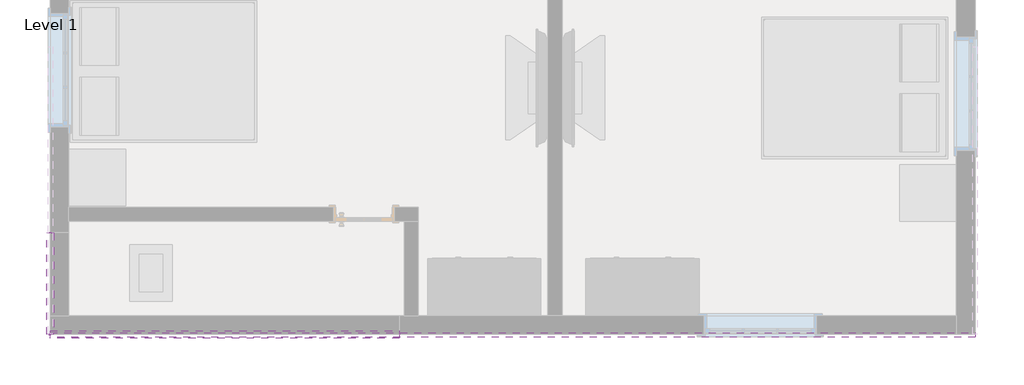
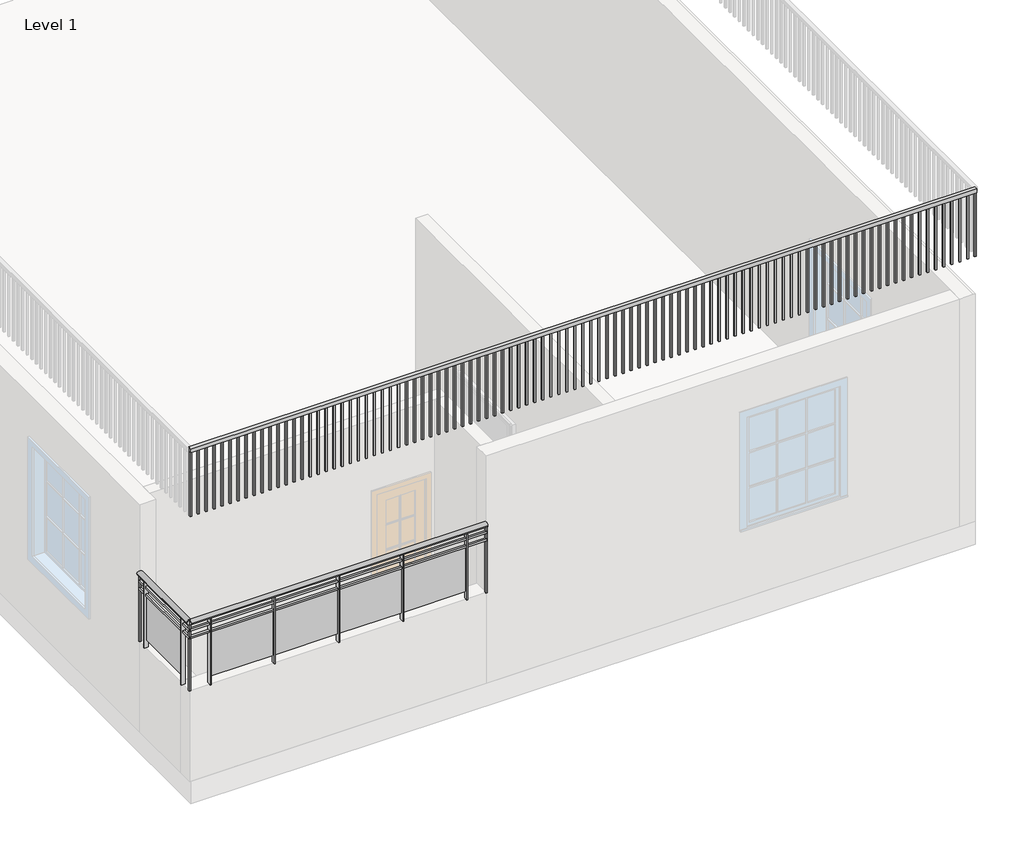
# One storey, part 2 of 7: 3 railings.
"""IFC4 building model written with IfcOpenShell, lengths in millimetres."""

from ifc_helpers import new_model, si_unit, point, frame, origin, place, context, project, spatial, polyline, ellipse_curve, trimmed, outline, extrude, element, save
from ifc_brep_helpers import plane_surface, extruded_surface, advanced_brep

model = new_model("IFC4")

# Units and contexts
model_context = context("Model", 3, world=origin())
ifc_project = project(units=[si_unit("LENGTHUNIT", "METRE", prefix="MILLI")], contexts=[model_context])

# Site, building, storey
site = spatial("IfcSite", under=ifc_project)
building = spatial("IfcBuilding", under=site)
storey = spatial("IfcBuildingStorey", under=building, Name="Level 1", Elevation=0.0)

# Railings
placement = place(None, origin())
element("IfcRailing", 1, ObjectType="Glass Panel - Bottom Fill", at=placement, inside=storey, context=model_context, shape_type="SolidModel", body=[
    advanced_brep(
    [(-8442.18475, -376.3160527, 2133.6), (-8518.38475, -376.3160527, 2133.6), (-8442.18475, -1468.5160527, 2133.6), (-8518.38475, -1468.5160527, 2133.6)],
    [
        (0, 1, ellipse_curve(frame((-8480.28475, -376.3160527, 2133.6), z_axis=(0.0, 1.0, 0.0), x_axis=(-1.0, 0.0, 0.0)), 38.1, 28.575)),
        (1, 0, ellipse_curve(frame((-8480.28475, -376.3160527, 2133.6), z_axis=(0.0, 1.0, 0.0), x_axis=(-1.0, 0.0, 0.0)), 38.1, 28.575)),
        (2, 3, ellipse_curve(frame((-8480.28475, -1468.5160527, 2133.6), z_axis=(0.0, -1.0, 0.0), x_axis=(-1.0, 0.0, 0.0)), 38.1, 28.575)),
        (3, 2, ellipse_curve(frame((-8480.28475, -1468.5160527, 2133.6), z_axis=(0.0, -1.0, 0.0), x_axis=(-1.0, 0.0, 0.0)), 38.1, 28.575)),
        (0, 2),
        (3, 1),
    ],
    [
        plane_surface(frame((-8480.28475, -376.3160527, 2133.6), z_axis=(0.0, 1.0, 0.0), x_axis=(0.0, 0.0, -1.0))),
        plane_surface(frame((-8480.28475, -1468.5160527, 2133.6), z_axis=(0.0, -1.0, 0.0), x_axis=(0.0, 0.0, -1.0))),
        extruded_surface(trimmed(ellipse_curve(frame((-8480.28475, -1468.5160527, 2133.6), z_axis=(0.0, 1.0, 0.0), x_axis=(-1.0, 0.0, 0.0)), 38.1, 28.575), [point((-8442.18475, -1468.5160527, 2133.6))], [point((-8518.38475, -1468.5160527, 2133.6))], True, "CARTESIAN"), (0.0, 1092.2, 0.0), 1092.2),
        extruded_surface(trimmed(ellipse_curve(frame((-8480.28475, -1468.5160527, 2133.6), z_axis=(0.0, 1.0, 0.0), x_axis=(-1.0, 0.0, 0.0)), 38.1, 28.575), [point((-8518.38475, -1468.5160527, 2133.6))], [point((-8442.18475, -1468.5160527, 2133.6))], True, "CARTESIAN"), (0.0, 1092.2, 0.0), 1092.2),
    ],
    [
        (0, [[1, 2]]),
        (1, [[3, 4]]),
        (2, [[-1, 5, -4, 6]]),
        (3, [[-2, -6, -3, -5]]),
    ],
),
    extrude(outline(polyline([(-8492.98475, -376.3160527), (-8467.58475, -376.3160527), (-8467.58475, -1468.5160527), (-8492.98475, -1468.5160527), (-8492.98475, -376.3160527)])), frame((0.0, 0.0, 2019.3), z_axis=(0.0, 0.0, 1.0), x_axis=(1.0, 0.0, 0.0)), (0.0, 0.0, 1.0), 25.4),
    extrude(outline(polyline([(-8492.98475, -376.3160527), (-8467.58475, -376.3160527), (-8467.58475, -1468.5160527), (-8492.98475, -1468.5160527), (-8492.98475, -376.3160527)])), frame((0.0, 0.0, 1917.7), z_axis=(0.0, 0.0, 1.0), x_axis=(1.0, 0.0, 0.0)), (0.0, 0.0, 1.0), 25.4),
    extrude(outline(polyline([(-8505.68475, -1322.4660527), (-8454.88475, -1322.4660527), (-8454.88475, -1335.1660527), (-8505.68475, -1335.1660527), (-8505.68475, -1322.4660527)])), frame((0.0, 0.0, 1219.2), z_axis=(0.0, 0.0, 1.0), x_axis=(1.0, 0.0, 0.0)), (0.0, 0.0, 1.0), 885.6788223),
    extrude(outline(polyline([(-8473.749593, -516.0160527), (-8473.749593, -1328.8160527), (-8480.099593, -1328.8160527), (-8480.099593, -516.0160527), (-8473.749593, -516.0160527)])), frame((0.0, 0.0, 1320.8), z_axis=(0.0, 0.0, 1.0), x_axis=(1.0, 0.0, 0.0)), (0.0, 0.0, 1.0), 596.9),
    extrude(outline(polyline([(-8505.68475, -509.6660527), (-8454.88475, -509.6660527), (-8454.88475, -522.3660527), (-8505.68475, -522.3660527), (-8505.68475, -509.6660527)])), frame((0.0, 0.0, 1219.2), z_axis=(0.0, 0.0, 1.0), x_axis=(1.0, 0.0, 0.0)), (0.0, 0.0, 1.0), 885.6788223),
    extrude(outline(polyline([(-8489.80975, -1455.8160527), (-8470.75975, -1455.8160527), (-8470.75975, -1474.8660527), (-8489.80975, -1474.8660527), (-8489.80975, -1455.8160527)])), frame((0.0, 0.0, 1219.2), z_axis=(0.0, 0.0, 1.0), x_axis=(1.0, 0.0, 0.0)), (0.0, 0.0, 1.0), 885.6788223),
    extrude(outline(polyline([(-8489.80975, -369.9660527), (-8470.75975, -369.9660527), (-8470.75975, -389.0160527), (-8489.80975, -389.0160527), (-8489.80975, -369.9660527)])), frame((0.0, 0.0, 1219.2), z_axis=(0.0, 0.0, 1.0), x_axis=(1.0, 0.0, 0.0)), (0.0, 0.0, 1.0), 885.6788223),
])
element("IfcRailing", 2, ObjectType="Glass Panel - Bottom Fill", at=placement, inside=storey, context=model_context, shape_type="SolidModel", body=[
    advanced_brep(
    [(-8480.28475, -1430.4160527, 2133.6), (-8480.28475, -1506.6160527, 2133.6), (-4721.08475, -1430.4160527, 2133.6), (-4721.08475, -1506.6160527, 2133.6)],
    [
        (0, 1, ellipse_curve(frame((-8480.28475, -1468.5160527, 2133.6), z_axis=(-1.0, 0.0, 0.0), x_axis=(0.0, -1.0, 0.0)), 38.1, 28.575)),
        (1, 0, ellipse_curve(frame((-8480.28475, -1468.5160527, 2133.6), z_axis=(-1.0, 0.0, 0.0), x_axis=(0.0, -1.0, 0.0)), 38.1, 28.575)),
        (2, 3, ellipse_curve(frame((-4721.08475, -1468.5160527, 2133.6), z_axis=(1.0, 0.0, 0.0), x_axis=(0.0, -1.0, 0.0)), 38.1, 28.575)),
        (3, 2, ellipse_curve(frame((-4721.08475, -1468.5160527, 2133.6), z_axis=(1.0, 0.0, 0.0), x_axis=(0.0, -1.0, 0.0)), 38.1, 28.575)),
        (0, 2),
        (3, 1),
    ],
    [
        plane_surface(frame((-8480.28475, -1468.5160527, 2133.6), z_axis=(-1.0, 0.0, 0.0), x_axis=(0.0, 1.0, 0.0))),
        plane_surface(frame((-4721.08475, -1468.5160527, 2133.6), z_axis=(1.0, 0.0, 0.0), x_axis=(0.0, 1.0, 0.0))),
        extruded_surface(trimmed(ellipse_curve(frame((-4721.08475, -1468.5160527, 2133.6), z_axis=(-1.0, 0.0, 0.0), x_axis=(0.0, -1.0, 0.0)), 38.1, 28.575), [point((-4721.08475, -1430.4160527, 2133.6))], [point((-4721.08475, -1506.6160527, 2133.6))], True, "CARTESIAN"), (-3759.2000000000007, 0.0, 0.0), 3759.2000000000007),
        extruded_surface(trimmed(ellipse_curve(frame((-4721.08475, -1468.5160527, 2133.6), z_axis=(-1.0, 0.0, 0.0), x_axis=(0.0, -1.0, 0.0)), 38.1, 28.575), [point((-4721.08475, -1506.6160527, 2133.6))], [point((-4721.08475, -1430.4160527, 2133.6))], True, "CARTESIAN"), (-3759.2000000000007, 0.0, 0.0), 3759.2000000000007),
    ],
    [
        (0, [[1, 2]]),
        (1, [[3, 4]]),
        (2, [[-1, 5, -4, 6]]),
        (3, [[-2, -6, -3, -5]]),
    ],
),
    extrude(outline(polyline([(-8480.28475, -1481.2160527), (-8480.28475, -1455.8160527), (-4721.08475, -1455.8160527), (-4721.08475, -1481.2160527), (-8480.28475, -1481.2160527)])), frame((0.0, 0.0, 2019.3), z_axis=(0.0, 0.0, 1.0), x_axis=(1.0, 0.0, 0.0)), (0.0, 0.0, 1.0), 25.4),
    extrude(outline(polyline([(-8480.28475, -1481.2160527), (-8480.28475, -1455.8160527), (-4721.08475, -1455.8160527), (-4721.08475, -1481.2160527), (-8480.28475, -1481.2160527)])), frame((0.0, 0.0, 1917.7), z_axis=(0.0, 0.0, 1.0), x_axis=(1.0, 0.0, 0.0)), (0.0, 0.0, 1.0), 25.4),
    extrude(outline(polyline([(-4981.43475, -1493.9160527), (-4981.43475, -1443.1160527), (-4968.73475, -1443.1160527), (-4968.73475, -1493.9160527), (-4981.43475, -1493.9160527)])), frame((0.0, 0.0, 1219.2), z_axis=(0.0, 0.0, 1.0), x_axis=(1.0, 0.0, 0.0)), (0.0, 0.0, 1.0), 885.6788223),
    extrude(outline(polyline([(-5787.88475, -1461.9808957), (-4975.08475, -1461.9808957), (-4975.08475, -1468.3308957), (-5787.88475, -1468.3308957), (-5787.88475, -1461.9808957)])), frame((0.0, 0.0, 1320.8), z_axis=(0.0, 0.0, 1.0), x_axis=(1.0, 0.0, 0.0)), (0.0, 0.0, 1.0), 596.9),
    extrude(outline(polyline([(-5794.23475, -1493.9160527), (-5794.23475, -1443.1160527), (-5781.53475, -1443.1160527), (-5781.53475, -1493.9160527), (-5794.23475, -1493.9160527)])), frame((0.0, 0.0, 1219.2), z_axis=(0.0, 0.0, 1.0), x_axis=(1.0, 0.0, 0.0)), (0.0, 0.0, 1.0), 885.6788223),
    extrude(outline(polyline([(-6600.68475, -1461.9808957), (-5787.88475, -1461.9808957), (-5787.88475, -1468.3308957), (-6600.68475, -1468.3308957), (-6600.68475, -1461.9808957)])), frame((0.0, 0.0, 1320.8), z_axis=(0.0, 0.0, 1.0), x_axis=(1.0, 0.0, 0.0)), (0.0, 0.0, 1.0), 596.9),
    extrude(outline(polyline([(-6607.03475, -1493.9160527), (-6607.03475, -1443.1160527), (-6594.33475, -1443.1160527), (-6594.33475, -1493.9160527), (-6607.03475, -1493.9160527)])), frame((0.0, 0.0, 1219.2), z_axis=(0.0, 0.0, 1.0), x_axis=(1.0, 0.0, 0.0)), (0.0, 0.0, 1.0), 885.6788223),
    extrude(outline(polyline([(-7413.48475, -1461.9808957), (-6600.68475, -1461.9808957), (-6600.68475, -1468.3308957), (-7413.48475, -1468.3308957), (-7413.48475, -1461.9808957)])), frame((0.0, 0.0, 1320.8), z_axis=(0.0, 0.0, 1.0), x_axis=(1.0, 0.0, 0.0)), (0.0, 0.0, 1.0), 596.9),
    extrude(outline(polyline([(-7419.83475, -1493.9160527), (-7419.83475, -1443.1160527), (-7407.13475, -1443.1160527), (-7407.13475, -1493.9160527), (-7419.83475, -1493.9160527)])), frame((0.0, 0.0, 1219.2), z_axis=(0.0, 0.0, 1.0), x_axis=(1.0, 0.0, 0.0)), (0.0, 0.0, 1.0), 885.6788223),
    extrude(outline(polyline([(-8226.28475, -1461.9808957), (-7413.48475, -1461.9808957), (-7413.48475, -1468.3308957), (-8226.28475, -1468.3308957), (-8226.28475, -1461.9808957)])), frame((0.0, 0.0, 1320.8), z_axis=(0.0, 0.0, 1.0), x_axis=(1.0, 0.0, 0.0)), (0.0, 0.0, 1.0), 596.9),
    extrude(outline(polyline([(-8232.63475, -1493.9160527), (-8232.63475, -1443.1160527), (-8219.93475, -1443.1160527), (-8219.93475, -1493.9160527), (-8232.63475, -1493.9160527)])), frame((0.0, 0.0, 1219.2), z_axis=(0.0, 0.0, 1.0), x_axis=(1.0, 0.0, 0.0)), (0.0, 0.0, 1.0), 885.6788223),
    extrude(outline(polyline([(-4733.78475, -1478.0410527), (-4733.78475, -1458.9910527), (-4714.73475, -1458.9910527), (-4714.73475, -1478.0410527), (-4733.78475, -1478.0410527)])), frame((0.0, 0.0, 1219.2), z_axis=(0.0, 0.0, 1.0), x_axis=(1.0, 0.0, 0.0)), (0.0, 0.0, 1.0), 885.6788223),
    extrude(outline(polyline([(-8486.63475, -1478.0410527), (-8486.63475, -1458.9910527), (-8467.58475, -1458.9910527), (-8467.58475, -1478.0410527), (-8486.63475, -1478.0410527)])), frame((0.0, 0.0, 1219.2), z_axis=(0.0, 0.0, 1.0), x_axis=(1.0, 0.0, 0.0)), (0.0, 0.0, 1.0), 885.6788223),
])
element("IfcRailing", 3, ObjectType="Handrail - Rectangular", at=placement, inside=storey, context=model_context, shape_type="SweptSolid", body=[
    extrude(outline(polyline([(-8480.28475, -1500.2660527), (-8480.28475, -1449.4660527), (1476.51525, -1449.4660527), (1476.51525, -1500.2660527), (-8480.28475, -1500.2660527)])), frame((0.0, 0.0, 4419.6), z_axis=(0.0, 0.0, 1.0), x_axis=(1.0, 0.0, 0.0)), (0.0, 0.0, 1.0), 50.8),
    extrude(outline(polyline([(1365.39025, -1484.3910527), (1365.39025, -1465.3410527), (1384.44025, -1465.3410527), (1384.44025, -1484.3910527), (1365.39025, -1484.3910527)])), frame((0.0, 0.0, 3556.0), z_axis=(0.0, 0.0, 1.0), x_axis=(1.0, 0.0, 0.0)), (0.0, 0.0, 1.0), 863.6),
    extrude(outline(polyline([(1263.79025, -1484.3910527), (1263.79025, -1465.3410527), (1282.84025, -1465.3410527), (1282.84025, -1484.3910527), (1263.79025, -1484.3910527)])), frame((0.0, 0.0, 3556.0), z_axis=(0.0, 0.0, 1.0), x_axis=(1.0, 0.0, 0.0)), (0.0, 0.0, 1.0), 863.6),
    extrude(outline(polyline([(1162.19025, -1484.3910527), (1162.19025, -1465.3410527), (1181.24025, -1465.3410527), (1181.24025, -1484.3910527), (1162.19025, -1484.3910527)])), frame((0.0, 0.0, 3556.0), z_axis=(0.0, 0.0, 1.0), x_axis=(1.0, 0.0, 0.0)), (0.0, 0.0, 1.0), 863.6),
    extrude(outline(polyline([(1060.59025, -1484.3910527), (1060.59025, -1465.3410527), (1079.64025, -1465.3410527), (1079.64025, -1484.3910527), (1060.59025, -1484.3910527)])), frame((0.0, 0.0, 3556.0), z_axis=(0.0, 0.0, 1.0), x_axis=(1.0, 0.0, 0.0)), (0.0, 0.0, 1.0), 863.6),
    extrude(outline(polyline([(958.99025, -1484.3910527), (958.99025, -1465.3410527), (978.04025, -1465.3410527), (978.04025, -1484.3910527), (958.99025, -1484.3910527)])), frame((0.0, 0.0, 3556.0), z_axis=(0.0, 0.0, 1.0), x_axis=(1.0, 0.0, 0.0)), (0.0, 0.0, 1.0), 863.6),
    extrude(outline(polyline([(857.39025, -1484.3910527), (857.39025, -1465.3410527), (876.44025, -1465.3410527), (876.44025, -1484.3910527), (857.39025, -1484.3910527)])), frame((0.0, 0.0, 3556.0), z_axis=(0.0, 0.0, 1.0), x_axis=(1.0, 0.0, 0.0)), (0.0, 0.0, 1.0), 863.6),
    extrude(outline(polyline([(755.79025, -1484.3910527), (755.79025, -1465.3410527), (774.84025, -1465.3410527), (774.84025, -1484.3910527), (755.79025, -1484.3910527)])), frame((0.0, 0.0, 3556.0), z_axis=(0.0, 0.0, 1.0), x_axis=(1.0, 0.0, 0.0)), (0.0, 0.0, 1.0), 863.6),
    extrude(outline(polyline([(654.19025, -1484.3910527), (654.19025, -1465.3410527), (673.24025, -1465.3410527), (673.24025, -1484.3910527), (654.19025, -1484.3910527)])), frame((0.0, 0.0, 3556.0), z_axis=(0.0, 0.0, 1.0), x_axis=(1.0, 0.0, 0.0)), (0.0, 0.0, 1.0), 863.6),
    extrude(outline(polyline([(552.59025, -1484.3910527), (552.59025, -1465.3410527), (571.64025, -1465.3410527), (571.64025, -1484.3910527), (552.59025, -1484.3910527)])), frame((0.0, 0.0, 3556.0), z_axis=(0.0, 0.0, 1.0), x_axis=(1.0, 0.0, 0.0)), (0.0, 0.0, 1.0), 863.6),
    extrude(outline(polyline([(450.99025, -1484.3910527), (450.99025, -1465.3410527), (470.04025, -1465.3410527), (470.04025, -1484.3910527), (450.99025, -1484.3910527)])), frame((0.0, 0.0, 3556.0), z_axis=(0.0, 0.0, 1.0), x_axis=(1.0, 0.0, 0.0)), (0.0, 0.0, 1.0), 863.6),
    extrude(outline(polyline([(349.39025, -1484.3910527), (349.39025, -1465.3410527), (368.44025, -1465.3410527), (368.44025, -1484.3910527), (349.39025, -1484.3910527)])), frame((0.0, 0.0, 3556.0), z_axis=(0.0, 0.0, 1.0), x_axis=(1.0, 0.0, 0.0)), (0.0, 0.0, 1.0), 863.6),
    extrude(outline(polyline([(247.79025, -1484.3910527), (247.79025, -1465.3410527), (266.84025, -1465.3410527), (266.84025, -1484.3910527), (247.79025, -1484.3910527)])), frame((0.0, 0.0, 3556.0), z_axis=(0.0, 0.0, 1.0), x_axis=(1.0, 0.0, 0.0)), (0.0, 0.0, 1.0), 863.6),
    extrude(outline(polyline([(146.19025, -1484.3910527), (146.19025, -1465.3410527), (165.24025, -1465.3410527), (165.24025, -1484.3910527), (146.19025, -1484.3910527)])), frame((0.0, 0.0, 3556.0), z_axis=(0.0, 0.0, 1.0), x_axis=(1.0, 0.0, 0.0)), (0.0, 0.0, 1.0), 863.6),
    extrude(outline(polyline([(44.59025, -1484.3910527), (44.59025, -1465.3410527), (63.64025, -1465.3410527), (63.64025, -1484.3910527), (44.59025, -1484.3910527)])), frame((0.0, 0.0, 3556.0), z_axis=(0.0, 0.0, 1.0), x_axis=(1.0, 0.0, 0.0)), (0.0, 0.0, 1.0), 863.6),
    extrude(outline(polyline([(-57.00975, -1484.3910527), (-57.00975, -1465.3410527), (-37.95975, -1465.3410527), (-37.95975, -1484.3910527), (-57.00975, -1484.3910527)])), frame((0.0, 0.0, 3556.0), z_axis=(0.0, 0.0, 1.0), x_axis=(1.0, 0.0, 0.0)), (0.0, 0.0, 1.0), 863.6),
    extrude(outline(polyline([(-158.60975, -1484.3910527), (-158.60975, -1465.3410527), (-139.55975, -1465.3410527), (-139.55975, -1484.3910527), (-158.60975, -1484.3910527)])), frame((0.0, 0.0, 3556.0), z_axis=(0.0, 0.0, 1.0), x_axis=(1.0, 0.0, 0.0)), (0.0, 0.0, 1.0), 863.6),
    extrude(outline(polyline([(-260.20975, -1484.3910527), (-260.20975, -1465.3410527), (-241.15975, -1465.3410527), (-241.15975, -1484.3910527), (-260.20975, -1484.3910527)])), frame((0.0, 0.0, 3556.0), z_axis=(0.0, 0.0, 1.0), x_axis=(1.0, 0.0, 0.0)), (0.0, 0.0, 1.0), 863.6),
    extrude(outline(polyline([(-361.80975, -1484.3910527), (-361.80975, -1465.3410527), (-342.75975, -1465.3410527), (-342.75975, -1484.3910527), (-361.80975, -1484.3910527)])), frame((0.0, 0.0, 3556.0), z_axis=(0.0, 0.0, 1.0), x_axis=(1.0, 0.0, 0.0)), (0.0, 0.0, 1.0), 863.6),
    extrude(outline(polyline([(-463.40975, -1484.3910527), (-463.40975, -1465.3410527), (-444.35975, -1465.3410527), (-444.35975, -1484.3910527), (-463.40975, -1484.3910527)])), frame((0.0, 0.0, 3556.0), z_axis=(0.0, 0.0, 1.0), x_axis=(1.0, 0.0, 0.0)), (0.0, 0.0, 1.0), 863.6),
    extrude(outline(polyline([(-565.00975, -1484.3910527), (-565.00975, -1465.3410527), (-545.95975, -1465.3410527), (-545.95975, -1484.3910527), (-565.00975, -1484.3910527)])), frame((0.0, 0.0, 3556.0), z_axis=(0.0, 0.0, 1.0), x_axis=(1.0, 0.0, 0.0)), (0.0, 0.0, 1.0), 863.6),
    extrude(outline(polyline([(-666.60975, -1484.3910527), (-666.60975, -1465.3410527), (-647.55975, -1465.3410527), (-647.55975, -1484.3910527), (-666.60975, -1484.3910527)])), frame((0.0, 0.0, 3556.0), z_axis=(0.0, 0.0, 1.0), x_axis=(1.0, 0.0, 0.0)), (0.0, 0.0, 1.0), 863.6),
    extrude(outline(polyline([(-768.20975, -1484.3910527), (-768.20975, -1465.3410527), (-749.15975, -1465.3410527), (-749.15975, -1484.3910527), (-768.20975, -1484.3910527)])), frame((0.0, 0.0, 3556.0), z_axis=(0.0, 0.0, 1.0), x_axis=(1.0, 0.0, 0.0)), (0.0, 0.0, 1.0), 863.6),
    extrude(outline(polyline([(-869.80975, -1484.3910527), (-869.80975, -1465.3410527), (-850.75975, -1465.3410527), (-850.75975, -1484.3910527), (-869.80975, -1484.3910527)])), frame((0.0, 0.0, 3556.0), z_axis=(0.0, 0.0, 1.0), x_axis=(1.0, 0.0, 0.0)), (0.0, 0.0, 1.0), 863.6),
    extrude(outline(polyline([(-971.40975, -1484.3910527), (-971.40975, -1465.3410527), (-952.35975, -1465.3410527), (-952.35975, -1484.3910527), (-971.40975, -1484.3910527)])), frame((0.0, 0.0, 3556.0), z_axis=(0.0, 0.0, 1.0), x_axis=(1.0, 0.0, 0.0)), (0.0, 0.0, 1.0), 863.6),
    extrude(outline(polyline([(-1073.00975, -1484.3910527), (-1073.00975, -1465.3410527), (-1053.95975, -1465.3410527), (-1053.95975, -1484.3910527), (-1073.00975, -1484.3910527)])), frame((0.0, 0.0, 3556.0), z_axis=(0.0, 0.0, 1.0), x_axis=(1.0, 0.0, 0.0)), (0.0, 0.0, 1.0), 863.6),
    extrude(outline(polyline([(-1174.60975, -1484.3910527), (-1174.60975, -1465.3410527), (-1155.55975, -1465.3410527), (-1155.55975, -1484.3910527), (-1174.60975, -1484.3910527)])), frame((0.0, 0.0, 3556.0), z_axis=(0.0, 0.0, 1.0), x_axis=(1.0, 0.0, 0.0)), (0.0, 0.0, 1.0), 863.6),
    extrude(outline(polyline([(-1276.20975, -1484.3910527), (-1276.20975, -1465.3410527), (-1257.15975, -1465.3410527), (-1257.15975, -1484.3910527), (-1276.20975, -1484.3910527)])), frame((0.0, 0.0, 3556.0), z_axis=(0.0, 0.0, 1.0), x_axis=(1.0, 0.0, 0.0)), (0.0, 0.0, 1.0), 863.6),
    extrude(outline(polyline([(-1377.80975, -1484.3910527), (-1377.80975, -1465.3410527), (-1358.75975, -1465.3410527), (-1358.75975, -1484.3910527), (-1377.80975, -1484.3910527)])), frame((0.0, 0.0, 3556.0), z_axis=(0.0, 0.0, 1.0), x_axis=(1.0, 0.0, 0.0)), (0.0, 0.0, 1.0), 863.6),
    extrude(outline(polyline([(-1479.40975, -1484.3910527), (-1479.40975, -1465.3410527), (-1460.35975, -1465.3410527), (-1460.35975, -1484.3910527), (-1479.40975, -1484.3910527)])), frame((0.0, 0.0, 3556.0), z_axis=(0.0, 0.0, 1.0), x_axis=(1.0, 0.0, 0.0)), (0.0, 0.0, 1.0), 863.6),
    extrude(outline(polyline([(-1581.00975, -1484.3910527), (-1581.00975, -1465.3410527), (-1561.95975, -1465.3410527), (-1561.95975, -1484.3910527), (-1581.00975, -1484.3910527)])), frame((0.0, 0.0, 3556.0), z_axis=(0.0, 0.0, 1.0), x_axis=(1.0, 0.0, 0.0)), (0.0, 0.0, 1.0), 863.6),
    extrude(outline(polyline([(-1682.60975, -1484.3910527), (-1682.60975, -1465.3410527), (-1663.55975, -1465.3410527), (-1663.55975, -1484.3910527), (-1682.60975, -1484.3910527)])), frame((0.0, 0.0, 3556.0), z_axis=(0.0, 0.0, 1.0), x_axis=(1.0, 0.0, 0.0)), (0.0, 0.0, 1.0), 863.6),
    extrude(outline(polyline([(-1784.20975, -1484.3910527), (-1784.20975, -1465.3410527), (-1765.15975, -1465.3410527), (-1765.15975, -1484.3910527), (-1784.20975, -1484.3910527)])), frame((0.0, 0.0, 3556.0), z_axis=(0.0, 0.0, 1.0), x_axis=(1.0, 0.0, 0.0)), (0.0, 0.0, 1.0), 863.6),
    extrude(outline(polyline([(-1885.80975, -1484.3910527), (-1885.80975, -1465.3410527), (-1866.75975, -1465.3410527), (-1866.75975, -1484.3910527), (-1885.80975, -1484.3910527)])), frame((0.0, 0.0, 3556.0), z_axis=(0.0, 0.0, 1.0), x_axis=(1.0, 0.0, 0.0)), (0.0, 0.0, 1.0), 863.6),
    extrude(outline(polyline([(-1987.40975, -1484.3910527), (-1987.40975, -1465.3410527), (-1968.35975, -1465.3410527), (-1968.35975, -1484.3910527), (-1987.40975, -1484.3910527)])), frame((0.0, 0.0, 3556.0), z_axis=(0.0, 0.0, 1.0), x_axis=(1.0, 0.0, 0.0)), (0.0, 0.0, 1.0), 863.6),
    extrude(outline(polyline([(-2089.00975, -1484.3910527), (-2089.00975, -1465.3410527), (-2069.95975, -1465.3410527), (-2069.95975, -1484.3910527), (-2089.00975, -1484.3910527)])), frame((0.0, 0.0, 3556.0), z_axis=(0.0, 0.0, 1.0), x_axis=(1.0, 0.0, 0.0)), (0.0, 0.0, 1.0), 863.6),
    extrude(outline(polyline([(-2190.60975, -1484.3910527), (-2190.60975, -1465.3410527), (-2171.55975, -1465.3410527), (-2171.55975, -1484.3910527), (-2190.60975, -1484.3910527)])), frame((0.0, 0.0, 3556.0), z_axis=(0.0, 0.0, 1.0), x_axis=(1.0, 0.0, 0.0)), (0.0, 0.0, 1.0), 863.6),
    extrude(outline(polyline([(-2292.20975, -1484.3910527), (-2292.20975, -1465.3410527), (-2273.15975, -1465.3410527), (-2273.15975, -1484.3910527), (-2292.20975, -1484.3910527)])), frame((0.0, 0.0, 3556.0), z_axis=(0.0, 0.0, 1.0), x_axis=(1.0, 0.0, 0.0)), (0.0, 0.0, 1.0), 863.6),
    extrude(outline(polyline([(-2393.80975, -1484.3910527), (-2393.80975, -1465.3410527), (-2374.75975, -1465.3410527), (-2374.75975, -1484.3910527), (-2393.80975, -1484.3910527)])), frame((0.0, 0.0, 3556.0), z_axis=(0.0, 0.0, 1.0), x_axis=(1.0, 0.0, 0.0)), (0.0, 0.0, 1.0), 863.6),
    extrude(outline(polyline([(-2495.40975, -1484.3910527), (-2495.40975, -1465.3410527), (-2476.35975, -1465.3410527), (-2476.35975, -1484.3910527), (-2495.40975, -1484.3910527)])), frame((0.0, 0.0, 3556.0), z_axis=(0.0, 0.0, 1.0), x_axis=(1.0, 0.0, 0.0)), (0.0, 0.0, 1.0), 863.6),
    extrude(outline(polyline([(-2597.00975, -1484.3910527), (-2597.00975, -1465.3410527), (-2577.95975, -1465.3410527), (-2577.95975, -1484.3910527), (-2597.00975, -1484.3910527)])), frame((0.0, 0.0, 3556.0), z_axis=(0.0, 0.0, 1.0), x_axis=(1.0, 0.0, 0.0)), (0.0, 0.0, 1.0), 863.6),
    extrude(outline(polyline([(-2698.60975, -1484.3910527), (-2698.60975, -1465.3410527), (-2679.55975, -1465.3410527), (-2679.55975, -1484.3910527), (-2698.60975, -1484.3910527)])), frame((0.0, 0.0, 3556.0), z_axis=(0.0, 0.0, 1.0), x_axis=(1.0, 0.0, 0.0)), (0.0, 0.0, 1.0), 863.6),
    extrude(outline(polyline([(-2800.20975, -1484.3910527), (-2800.20975, -1465.3410527), (-2781.15975, -1465.3410527), (-2781.15975, -1484.3910527), (-2800.20975, -1484.3910527)])), frame((0.0, 0.0, 3556.0), z_axis=(0.0, 0.0, 1.0), x_axis=(1.0, 0.0, 0.0)), (0.0, 0.0, 1.0), 863.6),
    extrude(outline(polyline([(-2901.80975, -1484.3910527), (-2901.80975, -1465.3410527), (-2882.75975, -1465.3410527), (-2882.75975, -1484.3910527), (-2901.80975, -1484.3910527)])), frame((0.0, 0.0, 3556.0), z_axis=(0.0, 0.0, 1.0), x_axis=(1.0, 0.0, 0.0)), (0.0, 0.0, 1.0), 863.6),
    extrude(outline(polyline([(-3003.40975, -1484.3910527), (-3003.40975, -1465.3410527), (-2984.35975, -1465.3410527), (-2984.35975, -1484.3910527), (-3003.40975, -1484.3910527)])), frame((0.0, 0.0, 3556.0), z_axis=(0.0, 0.0, 1.0), x_axis=(1.0, 0.0, 0.0)), (0.0, 0.0, 1.0), 863.6),
    extrude(outline(polyline([(-3105.00975, -1484.3910527), (-3105.00975, -1465.3410527), (-3085.95975, -1465.3410527), (-3085.95975, -1484.3910527), (-3105.00975, -1484.3910527)])), frame((0.0, 0.0, 3556.0), z_axis=(0.0, 0.0, 1.0), x_axis=(1.0, 0.0, 0.0)), (0.0, 0.0, 1.0), 863.6),
    extrude(outline(polyline([(-3206.60975, -1484.3910527), (-3206.60975, -1465.3410527), (-3187.55975, -1465.3410527), (-3187.55975, -1484.3910527), (-3206.60975, -1484.3910527)])), frame((0.0, 0.0, 3556.0), z_axis=(0.0, 0.0, 1.0), x_axis=(1.0, 0.0, 0.0)), (0.0, 0.0, 1.0), 863.6),
    extrude(outline(polyline([(-3308.20975, -1484.3910527), (-3308.20975, -1465.3410527), (-3289.15975, -1465.3410527), (-3289.15975, -1484.3910527), (-3308.20975, -1484.3910527)])), frame((0.0, 0.0, 3556.0), z_axis=(0.0, 0.0, 1.0), x_axis=(1.0, 0.0, 0.0)), (0.0, 0.0, 1.0), 863.6),
    extrude(outline(polyline([(-3409.80975, -1484.3910527), (-3409.80975, -1465.3410527), (-3390.75975, -1465.3410527), (-3390.75975, -1484.3910527), (-3409.80975, -1484.3910527)])), frame((0.0, 0.0, 3556.0), z_axis=(0.0, 0.0, 1.0), x_axis=(1.0, 0.0, 0.0)), (0.0, 0.0, 1.0), 863.6),
    extrude(outline(polyline([(-3511.40975, -1484.3910527), (-3511.40975, -1465.3410527), (-3492.35975, -1465.3410527), (-3492.35975, -1484.3910527), (-3511.40975, -1484.3910527)])), frame((0.0, 0.0, 3556.0), z_axis=(0.0, 0.0, 1.0), x_axis=(1.0, 0.0, 0.0)), (0.0, 0.0, 1.0), 863.6),
    extrude(outline(polyline([(-3613.00975, -1484.3910527), (-3613.00975, -1465.3410527), (-3593.95975, -1465.3410527), (-3593.95975, -1484.3910527), (-3613.00975, -1484.3910527)])), frame((0.0, 0.0, 3556.0), z_axis=(0.0, 0.0, 1.0), x_axis=(1.0, 0.0, 0.0)), (0.0, 0.0, 1.0), 863.6),
    extrude(outline(polyline([(-3714.60975, -1484.3910527), (-3714.60975, -1465.3410527), (-3695.55975, -1465.3410527), (-3695.55975, -1484.3910527), (-3714.60975, -1484.3910527)])), frame((0.0, 0.0, 3556.0), z_axis=(0.0, 0.0, 1.0), x_axis=(1.0, 0.0, 0.0)), (0.0, 0.0, 1.0), 863.6),
    extrude(outline(polyline([(-3816.20975, -1484.3910527), (-3816.20975, -1465.3410527), (-3797.15975, -1465.3410527), (-3797.15975, -1484.3910527), (-3816.20975, -1484.3910527)])), frame((0.0, 0.0, 3556.0), z_axis=(0.0, 0.0, 1.0), x_axis=(1.0, 0.0, 0.0)), (0.0, 0.0, 1.0), 863.6),
    extrude(outline(polyline([(-3917.80975, -1484.3910527), (-3917.80975, -1465.3410527), (-3898.75975, -1465.3410527), (-3898.75975, -1484.3910527), (-3917.80975, -1484.3910527)])), frame((0.0, 0.0, 3556.0), z_axis=(0.0, 0.0, 1.0), x_axis=(1.0, 0.0, 0.0)), (0.0, 0.0, 1.0), 863.6),
    extrude(outline(polyline([(-4019.40975, -1484.3910527), (-4019.40975, -1465.3410527), (-4000.35975, -1465.3410527), (-4000.35975, -1484.3910527), (-4019.40975, -1484.3910527)])), frame((0.0, 0.0, 3556.0), z_axis=(0.0, 0.0, 1.0), x_axis=(1.0, 0.0, 0.0)), (0.0, 0.0, 1.0), 863.6),
    extrude(outline(polyline([(-4121.00975, -1484.3910527), (-4121.00975, -1465.3410527), (-4101.95975, -1465.3410527), (-4101.95975, -1484.3910527), (-4121.00975, -1484.3910527)])), frame((0.0, 0.0, 3556.0), z_axis=(0.0, 0.0, 1.0), x_axis=(1.0, 0.0, 0.0)), (0.0, 0.0, 1.0), 863.6),
    extrude(outline(polyline([(-4222.60975, -1484.3910527), (-4222.60975, -1465.3410527), (-4203.55975, -1465.3410527), (-4203.55975, -1484.3910527), (-4222.60975, -1484.3910527)])), frame((0.0, 0.0, 3556.0), z_axis=(0.0, 0.0, 1.0), x_axis=(1.0, 0.0, 0.0)), (0.0, 0.0, 1.0), 863.6),
    extrude(outline(polyline([(-4324.20975, -1484.3910527), (-4324.20975, -1465.3410527), (-4305.15975, -1465.3410527), (-4305.15975, -1484.3910527), (-4324.20975, -1484.3910527)])), frame((0.0, 0.0, 3556.0), z_axis=(0.0, 0.0, 1.0), x_axis=(1.0, 0.0, 0.0)), (0.0, 0.0, 1.0), 863.6),
    extrude(outline(polyline([(-4425.80975, -1484.3910527), (-4425.80975, -1465.3410527), (-4406.75975, -1465.3410527), (-4406.75975, -1484.3910527), (-4425.80975, -1484.3910527)])), frame((0.0, 0.0, 3556.0), z_axis=(0.0, 0.0, 1.0), x_axis=(1.0, 0.0, 0.0)), (0.0, 0.0, 1.0), 863.6),
    extrude(outline(polyline([(-4527.40975, -1484.3910527), (-4527.40975, -1465.3410527), (-4508.35975, -1465.3410527), (-4508.35975, -1484.3910527), (-4527.40975, -1484.3910527)])), frame((0.0, 0.0, 3556.0), z_axis=(0.0, 0.0, 1.0), x_axis=(1.0, 0.0, 0.0)), (0.0, 0.0, 1.0), 863.6),
    extrude(outline(polyline([(-4629.00975, -1484.3910527), (-4629.00975, -1465.3410527), (-4609.95975, -1465.3410527), (-4609.95975, -1484.3910527), (-4629.00975, -1484.3910527)])), frame((0.0, 0.0, 3556.0), z_axis=(0.0, 0.0, 1.0), x_axis=(1.0, 0.0, 0.0)), (0.0, 0.0, 1.0), 863.6),
    extrude(outline(polyline([(-4730.60975, -1484.3910527), (-4730.60975, -1465.3410527), (-4711.55975, -1465.3410527), (-4711.55975, -1484.3910527), (-4730.60975, -1484.3910527)])), frame((0.0, 0.0, 3556.0), z_axis=(0.0, 0.0, 1.0), x_axis=(1.0, 0.0, 0.0)), (0.0, 0.0, 1.0), 863.6),
    extrude(outline(polyline([(-4832.20975, -1484.3910527), (-4832.20975, -1465.3410527), (-4813.15975, -1465.3410527), (-4813.15975, -1484.3910527), (-4832.20975, -1484.3910527)])), frame((0.0, 0.0, 3556.0), z_axis=(0.0, 0.0, 1.0), x_axis=(1.0, 0.0, 0.0)), (0.0, 0.0, 1.0), 863.6),
    extrude(outline(polyline([(-4933.80975, -1484.3910527), (-4933.80975, -1465.3410527), (-4914.75975, -1465.3410527), (-4914.75975, -1484.3910527), (-4933.80975, -1484.3910527)])), frame((0.0, 0.0, 3556.0), z_axis=(0.0, 0.0, 1.0), x_axis=(1.0, 0.0, 0.0)), (0.0, 0.0, 1.0), 863.6),
    extrude(outline(polyline([(-5035.40975, -1484.3910527), (-5035.40975, -1465.3410527), (-5016.35975, -1465.3410527), (-5016.35975, -1484.3910527), (-5035.40975, -1484.3910527)])), frame((0.0, 0.0, 3556.0), z_axis=(0.0, 0.0, 1.0), x_axis=(1.0, 0.0, 0.0)), (0.0, 0.0, 1.0), 863.6),
    extrude(outline(polyline([(-5137.00975, -1484.3910527), (-5137.00975, -1465.3410527), (-5117.95975, -1465.3410527), (-5117.95975, -1484.3910527), (-5137.00975, -1484.3910527)])), frame((0.0, 0.0, 3556.0), z_axis=(0.0, 0.0, 1.0), x_axis=(1.0, 0.0, 0.0)), (0.0, 0.0, 1.0), 863.6),
    extrude(outline(polyline([(-5238.60975, -1484.3910527), (-5238.60975, -1465.3410527), (-5219.55975, -1465.3410527), (-5219.55975, -1484.3910527), (-5238.60975, -1484.3910527)])), frame((0.0, 0.0, 3556.0), z_axis=(0.0, 0.0, 1.0), x_axis=(1.0, 0.0, 0.0)), (0.0, 0.0, 1.0), 863.6),
    extrude(outline(polyline([(-5340.20975, -1484.3910527), (-5340.20975, -1465.3410527), (-5321.15975, -1465.3410527), (-5321.15975, -1484.3910527), (-5340.20975, -1484.3910527)])), frame((0.0, 0.0, 3556.0), z_axis=(0.0, 0.0, 1.0), x_axis=(1.0, 0.0, 0.0)), (0.0, 0.0, 1.0), 863.6),
    extrude(outline(polyline([(-5441.80975, -1484.3910527), (-5441.80975, -1465.3410527), (-5422.75975, -1465.3410527), (-5422.75975, -1484.3910527), (-5441.80975, -1484.3910527)])), frame((0.0, 0.0, 3556.0), z_axis=(0.0, 0.0, 1.0), x_axis=(1.0, 0.0, 0.0)), (0.0, 0.0, 1.0), 863.6),
    extrude(outline(polyline([(-5543.40975, -1484.3910527), (-5543.40975, -1465.3410527), (-5524.35975, -1465.3410527), (-5524.35975, -1484.3910527), (-5543.40975, -1484.3910527)])), frame((0.0, 0.0, 3556.0), z_axis=(0.0, 0.0, 1.0), x_axis=(1.0, 0.0, 0.0)), (0.0, 0.0, 1.0), 863.6),
    extrude(outline(polyline([(-5645.00975, -1484.3910527), (-5645.00975, -1465.3410527), (-5625.95975, -1465.3410527), (-5625.95975, -1484.3910527), (-5645.00975, -1484.3910527)])), frame((0.0, 0.0, 3556.0), z_axis=(0.0, 0.0, 1.0), x_axis=(1.0, 0.0, 0.0)), (0.0, 0.0, 1.0), 863.6),
    extrude(outline(polyline([(-5746.60975, -1484.3910527), (-5746.60975, -1465.3410527), (-5727.55975, -1465.3410527), (-5727.55975, -1484.3910527), (-5746.60975, -1484.3910527)])), frame((0.0, 0.0, 3556.0), z_axis=(0.0, 0.0, 1.0), x_axis=(1.0, 0.0, 0.0)), (0.0, 0.0, 1.0), 863.6),
    extrude(outline(polyline([(-5848.20975, -1484.3910527), (-5848.20975, -1465.3410527), (-5829.15975, -1465.3410527), (-5829.15975, -1484.3910527), (-5848.20975, -1484.3910527)])), frame((0.0, 0.0, 3556.0), z_axis=(0.0, 0.0, 1.0), x_axis=(1.0, 0.0, 0.0)), (0.0, 0.0, 1.0), 863.6),
    extrude(outline(polyline([(-5949.80975, -1484.3910527), (-5949.80975, -1465.3410527), (-5930.75975, -1465.3410527), (-5930.75975, -1484.3910527), (-5949.80975, -1484.3910527)])), frame((0.0, 0.0, 3556.0), z_axis=(0.0, 0.0, 1.0), x_axis=(1.0, 0.0, 0.0)), (0.0, 0.0, 1.0), 863.6),
    extrude(outline(polyline([(-6051.40975, -1484.3910527), (-6051.40975, -1465.3410527), (-6032.35975, -1465.3410527), (-6032.35975, -1484.3910527), (-6051.40975, -1484.3910527)])), frame((0.0, 0.0, 3556.0), z_axis=(0.0, 0.0, 1.0), x_axis=(1.0, 0.0, 0.0)), (0.0, 0.0, 1.0), 863.6),
    extrude(outline(polyline([(-6153.00975, -1484.3910527), (-6153.00975, -1465.3410527), (-6133.95975, -1465.3410527), (-6133.95975, -1484.3910527), (-6153.00975, -1484.3910527)])), frame((0.0, 0.0, 3556.0), z_axis=(0.0, 0.0, 1.0), x_axis=(1.0, 0.0, 0.0)), (0.0, 0.0, 1.0), 863.6),
    extrude(outline(polyline([(-6254.60975, -1484.3910527), (-6254.60975, -1465.3410527), (-6235.55975, -1465.3410527), (-6235.55975, -1484.3910527), (-6254.60975, -1484.3910527)])), frame((0.0, 0.0, 3556.0), z_axis=(0.0, 0.0, 1.0), x_axis=(1.0, 0.0, 0.0)), (0.0, 0.0, 1.0), 863.6),
    extrude(outline(polyline([(-6356.20975, -1484.3910527), (-6356.20975, -1465.3410527), (-6337.15975, -1465.3410527), (-6337.15975, -1484.3910527), (-6356.20975, -1484.3910527)])), frame((0.0, 0.0, 3556.0), z_axis=(0.0, 0.0, 1.0), x_axis=(1.0, 0.0, 0.0)), (0.0, 0.0, 1.0), 863.6),
    extrude(outline(polyline([(-6457.80975, -1484.3910527), (-6457.80975, -1465.3410527), (-6438.75975, -1465.3410527), (-6438.75975, -1484.3910527), (-6457.80975, -1484.3910527)])), frame((0.0, 0.0, 3556.0), z_axis=(0.0, 0.0, 1.0), x_axis=(1.0, 0.0, 0.0)), (0.0, 0.0, 1.0), 863.6),
    extrude(outline(polyline([(-6559.40975, -1484.3910527), (-6559.40975, -1465.3410527), (-6540.35975, -1465.3410527), (-6540.35975, -1484.3910527), (-6559.40975, -1484.3910527)])), frame((0.0, 0.0, 3556.0), z_axis=(0.0, 0.0, 1.0), x_axis=(1.0, 0.0, 0.0)), (0.0, 0.0, 1.0), 863.6),
    extrude(outline(polyline([(-6661.00975, -1484.3910527), (-6661.00975, -1465.3410527), (-6641.95975, -1465.3410527), (-6641.95975, -1484.3910527), (-6661.00975, -1484.3910527)])), frame((0.0, 0.0, 3556.0), z_axis=(0.0, 0.0, 1.0), x_axis=(1.0, 0.0, 0.0)), (0.0, 0.0, 1.0), 863.6),
    extrude(outline(polyline([(-6762.60975, -1484.3910527), (-6762.60975, -1465.3410527), (-6743.55975, -1465.3410527), (-6743.55975, -1484.3910527), (-6762.60975, -1484.3910527)])), frame((0.0, 0.0, 3556.0), z_axis=(0.0, 0.0, 1.0), x_axis=(1.0, 0.0, 0.0)), (0.0, 0.0, 1.0), 863.6),
    extrude(outline(polyline([(-6864.20975, -1484.3910527), (-6864.20975, -1465.3410527), (-6845.15975, -1465.3410527), (-6845.15975, -1484.3910527), (-6864.20975, -1484.3910527)])), frame((0.0, 0.0, 3556.0), z_axis=(0.0, 0.0, 1.0), x_axis=(1.0, 0.0, 0.0)), (0.0, 0.0, 1.0), 863.6),
    extrude(outline(polyline([(-6965.80975, -1484.3910527), (-6965.80975, -1465.3410527), (-6946.75975, -1465.3410527), (-6946.75975, -1484.3910527), (-6965.80975, -1484.3910527)])), frame((0.0, 0.0, 3556.0), z_axis=(0.0, 0.0, 1.0), x_axis=(1.0, 0.0, 0.0)), (0.0, 0.0, 1.0), 863.6),
    extrude(outline(polyline([(-7067.40975, -1484.3910527), (-7067.40975, -1465.3410527), (-7048.35975, -1465.3410527), (-7048.35975, -1484.3910527), (-7067.40975, -1484.3910527)])), frame((0.0, 0.0, 3556.0), z_axis=(0.0, 0.0, 1.0), x_axis=(1.0, 0.0, 0.0)), (0.0, 0.0, 1.0), 863.6),
    extrude(outline(polyline([(-7169.00975, -1484.3910527), (-7169.00975, -1465.3410527), (-7149.95975, -1465.3410527), (-7149.95975, -1484.3910527), (-7169.00975, -1484.3910527)])), frame((0.0, 0.0, 3556.0), z_axis=(0.0, 0.0, 1.0), x_axis=(1.0, 0.0, 0.0)), (0.0, 0.0, 1.0), 863.6),
    extrude(outline(polyline([(-7270.60975, -1484.3910527), (-7270.60975, -1465.3410527), (-7251.55975, -1465.3410527), (-7251.55975, -1484.3910527), (-7270.60975, -1484.3910527)])), frame((0.0, 0.0, 3556.0), z_axis=(0.0, 0.0, 1.0), x_axis=(1.0, 0.0, 0.0)), (0.0, 0.0, 1.0), 863.6),
    extrude(outline(polyline([(-7372.20975, -1484.3910527), (-7372.20975, -1465.3410527), (-7353.15975, -1465.3410527), (-7353.15975, -1484.3910527), (-7372.20975, -1484.3910527)])), frame((0.0, 0.0, 3556.0), z_axis=(0.0, 0.0, 1.0), x_axis=(1.0, 0.0, 0.0)), (0.0, 0.0, 1.0), 863.6),
    extrude(outline(polyline([(-7473.80975, -1484.3910527), (-7473.80975, -1465.3410527), (-7454.75975, -1465.3410527), (-7454.75975, -1484.3910527), (-7473.80975, -1484.3910527)])), frame((0.0, 0.0, 3556.0), z_axis=(0.0, 0.0, 1.0), x_axis=(1.0, 0.0, 0.0)), (0.0, 0.0, 1.0), 863.6),
    extrude(outline(polyline([(-7575.40975, -1484.3910527), (-7575.40975, -1465.3410527), (-7556.35975, -1465.3410527), (-7556.35975, -1484.3910527), (-7575.40975, -1484.3910527)])), frame((0.0, 0.0, 3556.0), z_axis=(0.0, 0.0, 1.0), x_axis=(1.0, 0.0, 0.0)), (0.0, 0.0, 1.0), 863.6),
    extrude(outline(polyline([(-7677.00975, -1484.3910527), (-7677.00975, -1465.3410527), (-7657.95975, -1465.3410527), (-7657.95975, -1484.3910527), (-7677.00975, -1484.3910527)])), frame((0.0, 0.0, 3556.0), z_axis=(0.0, 0.0, 1.0), x_axis=(1.0, 0.0, 0.0)), (0.0, 0.0, 1.0), 863.6),
    extrude(outline(polyline([(-7778.60975, -1484.3910527), (-7778.60975, -1465.3410527), (-7759.55975, -1465.3410527), (-7759.55975, -1484.3910527), (-7778.60975, -1484.3910527)])), frame((0.0, 0.0, 3556.0), z_axis=(0.0, 0.0, 1.0), x_axis=(1.0, 0.0, 0.0)), (0.0, 0.0, 1.0), 863.6),
    extrude(outline(polyline([(-7880.20975, -1484.3910527), (-7880.20975, -1465.3410527), (-7861.15975, -1465.3410527), (-7861.15975, -1484.3910527), (-7880.20975, -1484.3910527)])), frame((0.0, 0.0, 3556.0), z_axis=(0.0, 0.0, 1.0), x_axis=(1.0, 0.0, 0.0)), (0.0, 0.0, 1.0), 863.6),
    extrude(outline(polyline([(-7981.80975, -1484.3910527), (-7981.80975, -1465.3410527), (-7962.75975, -1465.3410527), (-7962.75975, -1484.3910527), (-7981.80975, -1484.3910527)])), frame((0.0, 0.0, 3556.0), z_axis=(0.0, 0.0, 1.0), x_axis=(1.0, 0.0, 0.0)), (0.0, 0.0, 1.0), 863.6),
    extrude(outline(polyline([(-8083.40975, -1484.3910527), (-8083.40975, -1465.3410527), (-8064.35975, -1465.3410527), (-8064.35975, -1484.3910527), (-8083.40975, -1484.3910527)])), frame((0.0, 0.0, 3556.0), z_axis=(0.0, 0.0, 1.0), x_axis=(1.0, 0.0, 0.0)), (0.0, 0.0, 1.0), 863.6),
    extrude(outline(polyline([(-8185.00975, -1484.3910527), (-8185.00975, -1465.3410527), (-8165.95975, -1465.3410527), (-8165.95975, -1484.3910527), (-8185.00975, -1484.3910527)])), frame((0.0, 0.0, 3556.0), z_axis=(0.0, 0.0, 1.0), x_axis=(1.0, 0.0, 0.0)), (0.0, 0.0, 1.0), 863.6),
    extrude(outline(polyline([(-8286.60975, -1484.3910527), (-8286.60975, -1465.3410527), (-8267.55975, -1465.3410527), (-8267.55975, -1484.3910527), (-8286.60975, -1484.3910527)])), frame((0.0, 0.0, 3556.0), z_axis=(0.0, 0.0, 1.0), x_axis=(1.0, 0.0, 0.0)), (0.0, 0.0, 1.0), 863.6),
    extrude(outline(polyline([(-8388.20975, -1484.3910527), (-8388.20975, -1465.3410527), (-8369.15975, -1465.3410527), (-8369.15975, -1484.3910527), (-8388.20975, -1484.3910527)])), frame((0.0, 0.0, 3556.0), z_axis=(0.0, 0.0, 1.0), x_axis=(1.0, 0.0, 0.0)), (0.0, 0.0, 1.0), 863.6),
    extrude(outline(polyline([(1457.46525, -1484.3910527), (1457.46525, -1465.3410527), (1476.51525, -1465.3410527), (1476.51525, -1484.3910527), (1457.46525, -1484.3910527)])), frame((0.0, 0.0, 3556.0), z_axis=(0.0, 0.0, 1.0), x_axis=(1.0, 0.0, 0.0)), (0.0, 0.0, 1.0), 863.6),
    extrude(outline(polyline([(-8480.28475, -1484.3910527), (-8480.28475, -1465.3410527), (-8461.23475, -1465.3410527), (-8461.23475, -1484.3910527), (-8480.28475, -1484.3910527)])), frame((0.0, 0.0, 3556.0), z_axis=(0.0, 0.0, 1.0), x_axis=(1.0, 0.0, 0.0)), (0.0, 0.0, 1.0), 863.6),
])

save(model, "model.ifc")

# Revit data of these elements
# Type "Glass Panel - Bottom Fill"
#   Assembly Code = "C2010400"
#   built-in parameter 1008612 = 0.0416667 (stored number, unit not read)
#   built-in parameter 1008611 = 0.0416667 (stored number, unit not read)
#   built-in parameter 1008609 = 0.333333 (stored number, unit not read)
#   built-in parameter 1008604 = 0.166667 (stored number, unit not read)
#   built-in parameter 1008603 = 0.166667 (stored number, unit not read)
#   Railing Height = 3' - 0"
#   built-in parameter 1008630 = 2
#   built-in parameter 1008610 = 2
#   built-in parameter 1008618 = Baluster - Square : 3/4"
# Type "Handrail - Rectangular"
#   Assembly Code = "C2010400"
#   built-in parameter 1008612 = 0.0416667 (stored number, unit not read)
#   built-in parameter 1008611 = 0.0416667 (stored number, unit not read)
#   built-in parameter 1008609 = 0.333333 (stored number, unit not read)
#   built-in parameter 1008604 = 0.166667 (stored number, unit not read)
#   built-in parameter 1008603 = 0.166667 (stored number, unit not read)
#   Railing Height = 3' - 0"
#   built-in parameter 1008630 = 2
#   built-in parameter 1008610 = 2
#   built-in parameter 1008618 = Baluster - Square : 3/4"
# Elements 1, 2 (IfcRailing, "Glass Panel - Bottom Fill")
#   built-in parameter 1008621 = 4 (stored number, unit not read)
#   Phase Created = New Construction
#   Materials on its faces: "Glass"
# Element 3 (IfcRailing, "Handrail - Rectangular")
#   built-in parameter 1008621 = 11.6667 (stored number, unit not read)
#   Phase Created = New Construction
# Materials
#   "Glass": class "Glass", colour RGB 0 128 192, transparency 0.75, Description = "Soda Lime Glass", Cost = 0
